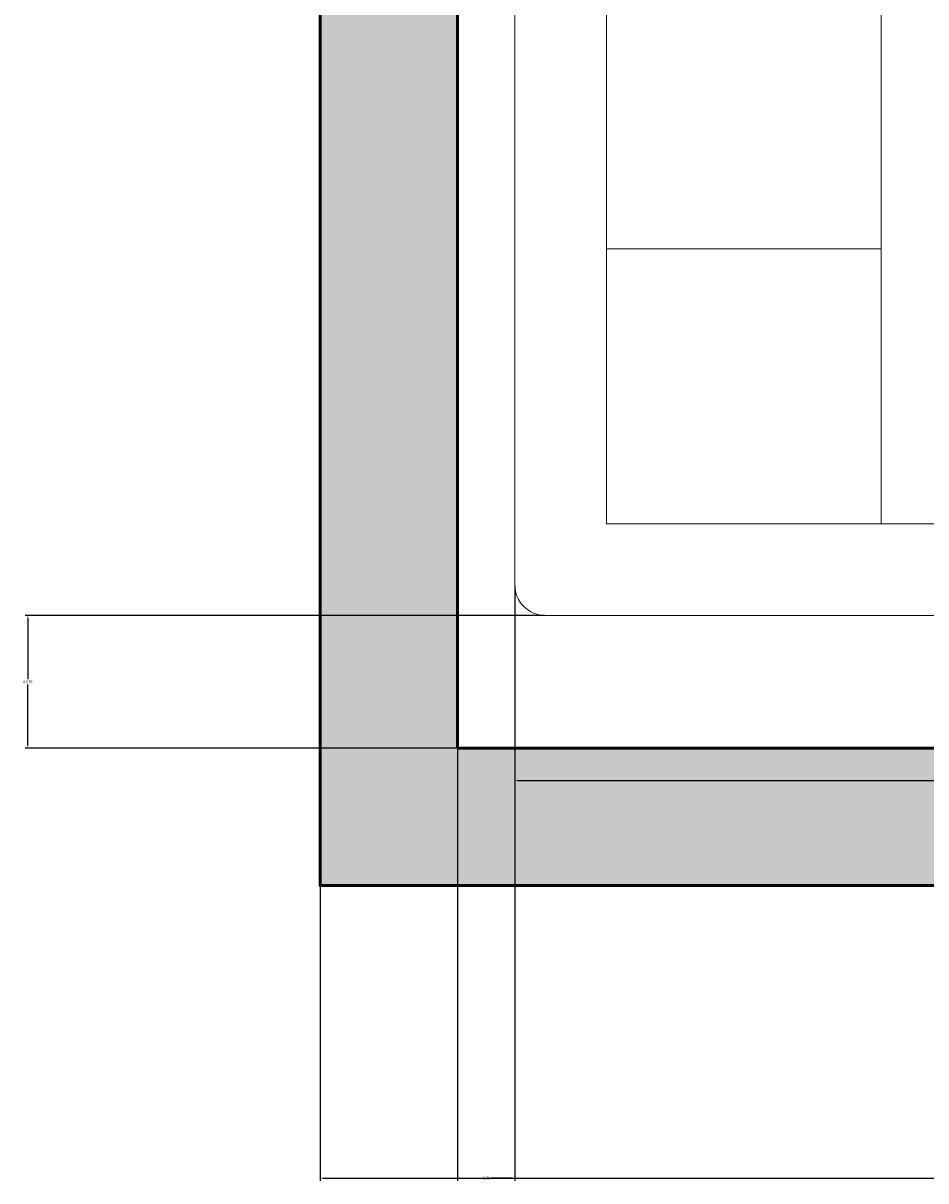
# Model space of a CAD drawing. Units: inches. Extents: x 2307 to 2544, y 2171 to 2540.
# Tile 1 of 52: x 2307 to 2366, y 2171 to 2247. Entities that reach past the tile are written whole.
import ezdxf

# ---------------------------------------------------------------- set-up
doc = ezdxf.new("R2010")
doc.units = ezdxf.units.IN
for name, color, linetype, lineweight in [('A-ANNO-DIMS', 2, 'Continuous', 18), ('A-FURN', 8, 'Continuous', 18), ('A-WALL', 7, 'Continuous', 50)]:
    doc.layers.add(name, color=color, linetype=linetype, lineweight=lineweight)
doc.layers.add('A-WALL-PATT', color=18, linetype='Continuous', lineweight=13, true_color=0x000000)
doc.styles.get("Standard").update_dxf_attribs({"font": 'arial.ttf'})
doc.dimstyles.get("Standard").update_dxf_attribs({"dimtxt": 0.18, "dimasz": 0.18, "dimexe": 0.18, "dimexo": 0.0625, "dimgap": 0.09, "dimtad": 0, "dimtih": 1, "dimtoh": 1, "dimdec": 4, "dimzin": 0, "dimdsep": 46, "dimtxsty": 'Standard', "dimcen": 0.09, "dimadec": 0, "dimazin": 0, "dimtfac": 1, "dimtdec": 4, "dimtofl": 0, "dimtmove": 0, "dimatfit": 3, "dimfxl": 1, "dimtolj": 1, "dimtzin": 0, "dimarcsym": 0})

# ---------------------------------------------------------------- blocks, each defined once
blk = doc.blocks.new('sofa')
for p, q in [((-21, 4), (-21, -64)), ((-15, -2), (-15, -60)), ((-15, -60), (9, -60)), ((-19, -66), (7, -66))]:
    blk.add_line(p, q)
for points in [[(3, -24), (-15, -24), (-15, -42), (3, -42)], [(3, -42), (-15, -42), (-15, -60), (3, -60)]]:
    blk.add_lwpolyline(points, close=True)
blk.add_arc((-19, -64), 2, 180, 270)
blk = doc.blocks.new('*D34')
at = {"layer": 'A-ANNO-DIMS', "color": 0, "lineweight": -2, "transparency": 16777216}
for p, q in [((2339.456, 2208.123), (2339.456, 2197.206)), ((2411.456, 2208.123), (2411.456, 2197.206)), ((2339.636, 2197.386), (2374.491, 2197.386)), ((2411.276, 2197.386), (2376.421, 2197.386))]:
    blk.add_line(p, q, dxfattribs=at)
at = {"layer": 'A-ANNO-DIMS', "color": 0, "transparency": 16777216}
for points in [[(2339.636, 2197.416), (2339.636, 2197.356), (2339.456, 2197.386)], [(2411.276, 2197.416), (2411.276, 2197.356), (2411.456, 2197.386)]]:
    blk.add_solid(points, dxfattribs=at)
at = {"layer": 'Defpoints', "color": 0, "transparency": 16777216}
for p in [(2339.456, 2208.186), (2411.456, 2208.186), (2411.456, 2197.386)]:
    blk.add_point(p, dxfattribs=at)
at = {"layer": 'A-ANNO-DIMS', "color": 0, "transparency": 16777216, "insert": (2375.456, 2197.386), "char_height": 0.18, "attachment_point": 5}
blk.add_mtext('\\A1;SECTIONAL 72', dxfattribs=at)
blk = doc.blocks.new('*D36')
at = {"layer": 'A-ANNO-DIMS', "color": 0, "lineweight": -2, "transparency": 16777216}
for p, q in [((2326.696, 2190.447), (2326.696, 2171.18)), ((2524.696, 2190.447), (2524.696, 2171.18)), ((2326.876, 2171.36), (2425.415, 2171.36)), ((2524.516, 2171.36), (2425.976, 2171.36))]:
    blk.add_line(p, q, dxfattribs=at)
at = {"layer": 'A-ANNO-DIMS', "color": 0, "transparency": 16777216}
for points in [[(2326.876, 2171.39), (2326.876, 2171.33), (2326.696, 2171.36)], [(2524.516, 2171.39), (2524.516, 2171.33), (2524.696, 2171.36)]]:
    blk.add_solid(points, dxfattribs=at)
at = {"layer": 'Defpoints', "color": 0, "transparency": 16777216}
for p in [(2326.696, 2190.51), (2524.696, 2190.51), (2524.696, 2171.36)]:
    blk.add_point(p, dxfattribs=at)
at = {"layer": 'A-ANNO-DIMS', "color": 0, "transparency": 16777216, "insert": (2425.696, 2171.36), "char_height": 0.18, "attachment_point": 5}
blk.add_mtext('\\A1;198', dxfattribs=at)
blk = doc.blocks.new('*D65')
at = {"layer": 'A-ANNO-DIMS', "color": 0, "lineweight": -2, "transparency": 16777216}
for p, q in [((2341.393, 2208.186), (2307.366, 2208.186)), ((2307.546, 2208.006), (2307.546, 2204.03)), ((2307.546, 2199.69), (2307.546, 2203.666)), ((2335.633, 2199.51), (2307.366, 2199.51))]:
    blk.add_line(p, q, dxfattribs=at)
at = {"layer": 'A-ANNO-DIMS', "color": 0, "transparency": 16777216}
for points in [[(2307.516, 2208.006), (2307.576, 2208.006), (2307.546, 2208.186)], [(2307.516, 2199.69), (2307.576, 2199.69), (2307.546, 2199.51)]]:
    blk.add_solid(points, dxfattribs=at)
at = {"layer": 'Defpoints', "color": 0, "transparency": 16777216}
for p in [(2307.546, 2208.186), (2341.456, 2208.186), (2335.696, 2199.51)]:
    blk.add_point(p, dxfattribs=at)
at = {"layer": 'A-ANNO-DIMS', "color": 0, "transparency": 16777216, "insert": (2307.546, 2203.848), "char_height": 0.18, "attachment_point": 5}
blk.add_mtext('\\A1;8.676', dxfattribs=at)
blk = doc.blocks.new('*D68')
at = {"layer": 'A-ANNO-DIMS', "color": 0, "lineweight": -2, "transparency": 16777216}
for p, q in [((2339.456, 2210.123), (2339.456, 2171.18)), ((2335.696, 2199.447), (2335.696, 2171.18)), ((2335.876, 2171.36), (2337.252, 2171.36)), ((2339.276, 2171.36), (2337.899, 2171.36))]:
    blk.add_line(p, q, dxfattribs=at)
at = {"layer": 'A-ANNO-DIMS', "color": 0, "transparency": 16777216}
for points in [[(2335.876, 2171.39), (2335.876, 2171.33), (2335.696, 2171.36)], [(2339.276, 2171.39), (2339.276, 2171.33), (2339.456, 2171.36)]]:
    blk.add_solid(points, dxfattribs=at)
at = {"layer": 'Defpoints', "color": 0, "transparency": 16777216}
for p in [(2339.456, 2210.186), (2335.696, 2199.51), (2339.456, 2171.36)]:
    blk.add_point(p, dxfattribs=at)
at = {"layer": 'A-ANNO-DIMS', "color": 0, "transparency": 16777216, "insert": (2337.576, 2171.36), "char_height": 0.18, "attachment_point": 5}
blk.add_mtext('\\A1;3.76', dxfattribs=at)

msp = doc.modelspace()

# ---------------------------------------------------------------- hatches: boundary and pattern name
at = {"layer": 'A-WALL-PATT'}
h = msp.add_hatch(color=256, dxfattribs=at)
h.dxf.hatch_style = 1
h.paths.add_polyline_path([(2433.6935, 2199.5096), (2415.6423, 2199.5096), (2415.6423, 2190.5096), (2433.7832, 2190.5096)], flags=17)
h.paths.add_polyline_path([(2367.6423, 2199.5096), (2335.6958, 2199.5096), (2335.6958, 2307.3983), (2326.6958, 2307.3983), (2326.6958, 2190.5096), (2367.6423, 2190.5096)])
h.paths.add_polyline_path([(2524.6958, 2520.5096), (2496.7832, 2520.5096), (2496.7832, 2515.5149), (2472.7832, 2515.5149), (2472.7832, 2520.5096), (2415.4028, 2520.5096), (2415.4028, 2511.5096), (2451.6958, 2511.5096), (2451.6958, 2439.5096), (2451.6958, 2391.5096), (2445.6958, 2391.5096), (2445.6958, 2387.5096), (2455.6958, 2387.5096), (2455.6958, 2435.5096), (2461.6958, 2435.5096), (2461.6958, 2439.5096), (2455.6958, 2439.5096), (2455.6958, 2511.5096), (2515.6958, 2511.5096), (2515.6958, 2439.5096), (2491.6958, 2439.5096), (2491.6958, 2435.5096), (2515.6958, 2435.5096), (2515.6958, 2319.5096), (2451.6958, 2319.5096), (2451.6958, 2281.5096), (2481.6958, 2281.5096), (2481.6958, 2225.5096), (2485.6958, 2225.5096), (2485.6958, 2285.5096), (2455.6958, 2285.5096), (2455.6958, 2315.5096), (2515.6958, 2315.5096), (2515.6958, 2199.5096), (2469.6952, 2199.5096), (2469.785, 2190.5096), (2524.6958, 2190.5096)])

# ---------------------------------------------------------------- linework, layer by layer
at = {"layer": 'A-WALL'}
for p, q in [((2335.6958, 2199.5096), (2335.6958, 2387.5096)), ((2433.6935, 2199.5096), (2335.6958, 2199.5096)), ((2433.6935, 2199.5096), (2335.6958, 2199.5096))]:
    msp.add_line(p, q, dxfattribs=at)
msp.add_lwpolyline([(2433.7832, 2190.5096), (2326.6958, 2190.5096), (2326.6958, 2520.5096), (2524.6958, 2520.5096), (2524.6958, 2190.5096), (2469.785, 2190.5096)], dxfattribs=at)

# ---------------------------------------------------------------- block references
at = {"layer": 'A-FURN'}
msp.add_blockref('sofa', (2360.4557, 2274.1858), dxfattribs=at)

# ---------------------------------------------------------------- dimensions: what is measured, and where the dimension line sits
at = {"layer": 'A-ANNO-DIMS'}
for base, p1, p2, override, picture, middle in [((2339.4557, 2171.3596), (2335.6958, 2199.5096), (2339.4557, 2210.1858), {"dimdec": 2, "dimlfac": 1, "dimrnd": 0, "dimzin": 0, "dimdsep": 46, "dimlunit": 2}, '*D68', (2337.5758, 2171.3596)), ((2524.6958, 2171.3596), (2326.6958, 2190.5096), (2524.6958, 2190.5096), {"dimdec": 0, "dimlfac": 1, "dimrnd": 0, "dimzin": 0, "dimdsep": 46, "dimlunit": 2}, '*D36', (2425.6958, 2171.3596))]:
    dim = msp.add_linear_dim(base=base, p1=p1, p2=p2, dimstyle='Standard', override=override, dxfattribs=at)
    dim.commit()
    dim.dimension.update_dxf_attribs({"geometry": picture, "text_midpoint": middle})
dim = msp.add_linear_dim(base=(2307.5458, 2208.1858), p1=(2335.6958, 2199.5096), p2=(2341.4557, 2208.1858), angle=90, dimstyle='Standard', override={"dimdec": 3, "dimlfac": 1, "dimrnd": 0, "dimzin": 0, "dimdsep": 46, "dimlunit": 2}, dxfattribs=at)
dim.commit()
dim.dimension.update_dxf_attribs({"geometry": '*D65', "text_midpoint": (2307.5458, 2203.8477)})
dim = msp.add_linear_dim(base=(2411.4557, 2197.3858), p1=(2339.4557, 2208.1858), p2=(2411.4557, 2208.1858), text='SECTIONAL <>', dimstyle='Standard', override={"dimdec": 0, "dimlfac": 1, "dimrnd": 0, "dimzin": 0, "dimdsep": 46, "dimlunit": 2}, dxfattribs=at)
dim.commit()
dim.dimension.update_dxf_attribs({"geometry": '*D34', "text_midpoint": (2375.4557, 2197.3858)})

doc.saveas('drawing.dxf')
